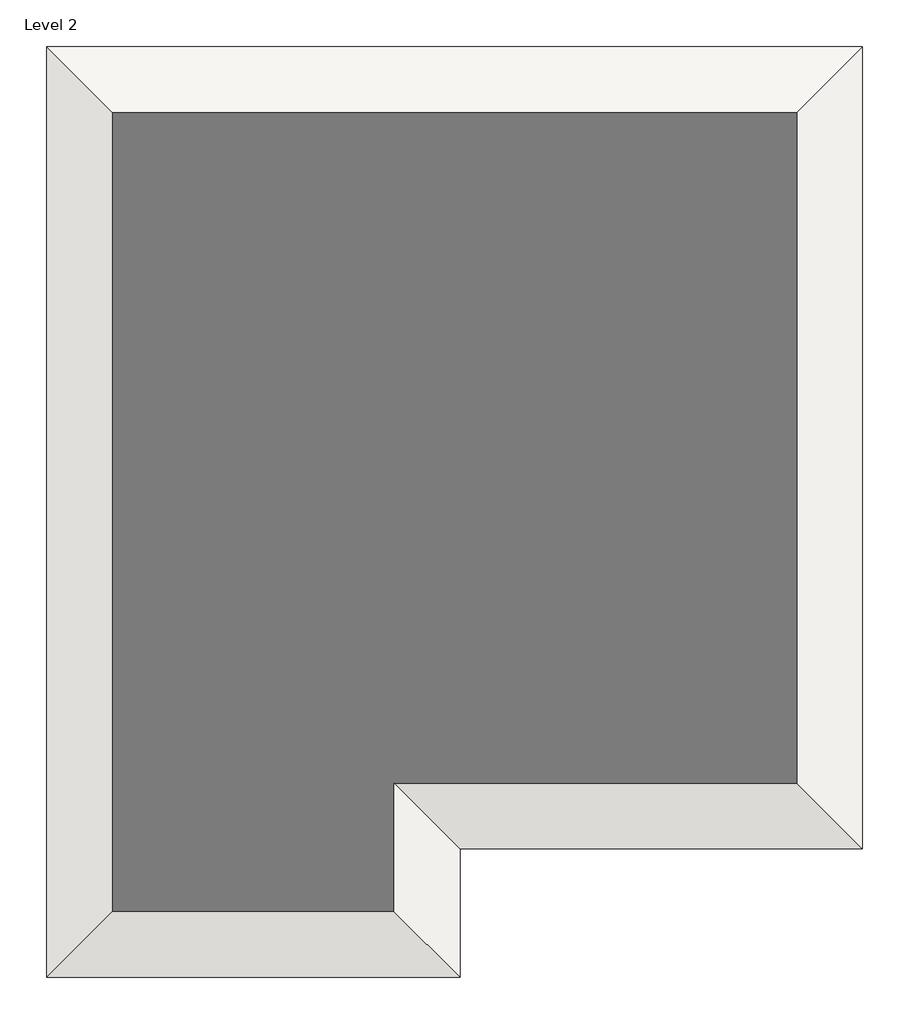
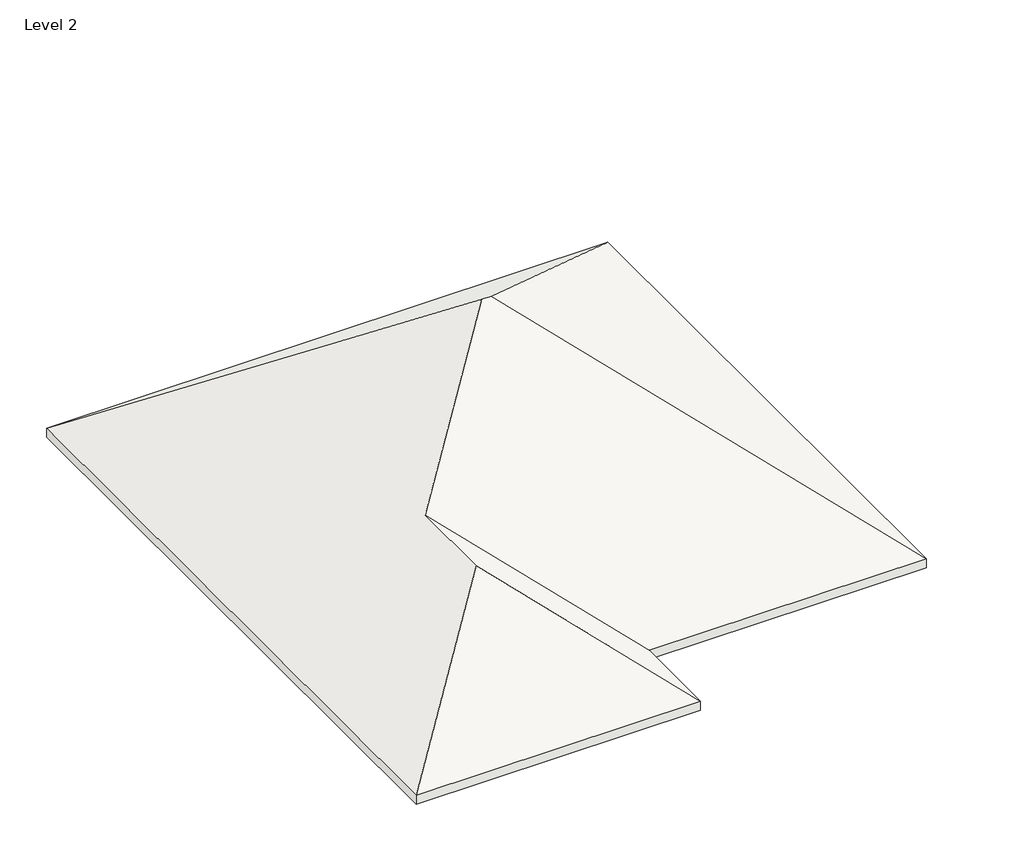
# One storey: 1 roof.
"""IFC4 building model written with IfcOpenShell, lengths in millimetres."""

from ifc_helpers import new_model, si_unit, origin, place, context, project, spatial, faceted_brep, element, save

model = new_model("IFC4")

# Units and contexts
model_context = context("Model", 3, world=origin())
ifc_project = project(units=[si_unit("LENGTHUNIT", "METRE", prefix="MILLI")], contexts=[model_context])

# Site, building, storey
site = spatial("IfcSite", under=ifc_project)
building = spatial("IfcBuilding", under=site)
storey = spatial("IfcBuildingStorey", under=building, Name="Level 2", Elevation=3048.0)

# Roof
placement = place(None, origin())
element("IfcRoof", 1, ObjectType="Wood Rafter 8\" - Asphalt Shingle - Insulated", at=placement, inside=storey, context=model_context, shape_type="Brep", body=[
    faceted_brep([(-9212.4392853, 5944.3049175, 8748.7125), (-1611.4892853, 13545.2549175, 3048.0), (-1611.4892853, -1656.6450825, 3048.0), (-17080.0892853, -4095.0450825, 3048.0), (-13162.1392853, -177.0950825, 5986.4625), (-9244.1892853, -4095.0450825, 3048.0), (-9479.1392853, 5944.3049175, 8748.7125), (-17080.0892853, 13545.2549175, 3048.0), (-9244.1892853, -1656.6450825, 3048.0), (-13162.1392853, 2261.3049175, 5986.4625), (-1611.4892853, 13545.2549175, 3313.90625), (-9212.4392853, 5944.3049175, 9014.61875), (-1611.4892853, -1656.6450825, 3313.90625), (-17080.0892853, -4095.0450825, 3313.90625), (-9244.1892853, -4095.0450825, 3313.90625), (-13162.1392853, -177.0950825, 6252.36875), (-17080.0892853, 13545.2549175, 3313.90625), (-9479.1392853, 5944.3049175, 9014.61875), (-9244.1892853, -1656.6450825, 3313.90625), (-13162.1392853, 2261.3049175, 6252.36875)], [[[0, 1, 2]], [[3, 4, 5]], [[1, 0, 6, 7]], [[8, 9, 6, 0, 2]], [[7, 6, 9, 4, 3]], [[8, 5, 4, 9]], [[10, 11, 12]], [[13, 14, 15]], [[10, 16, 17, 11]], [[18, 12, 11, 17, 19]], [[16, 13, 15, 19, 17]], [[14, 18, 19, 15]], [[7, 16, 10, 1]], [[3, 13, 16, 7]], [[5, 14, 13, 3]], [[8, 18, 14, 5]], [[2, 12, 18, 8]], [[1, 10, 12, 2]]]),
])

save(model, "model.ifc")

# Revit data of these elements
# Type "Wood Rafter 8\" - Asphalt Shingle - Insulated"
#   Assembly Code = "B1020"
#   Layers, outside or top first: 0' - 0 1/4" "Asphalt Shingle" (function 4); 0' - 0 5/8" "Plywood, Sheathing" (function 2); 0' - 7 1/2" "Structure, Wood Joist/Rafter Layer, Batt Insulation" (function 1)
# Element 1 (IfcRoof, "Wood Rafter 8\" - Asphalt Shingle - Insulated")
#   built-in parameter 1001705 = 29.5755 (stored number, unit not read)
#   built-in parameter 1001710 = 33615
#   Phase Created = New Construction
#   Materials on its faces: "Structure, Wood Joist/Rafter Layer, Batt Insulation", "Asphalt Shingle"
# Materials
#   "Asphalt Shingle": class "Generic", colour RGB 155 155 155, transparency 0, Description = "Asphalt roofing shingle", Cost = 0
#   "Plywood, Sheathing": class "Wood", colour RGB 212 179 113, transparency 0, Description = "Plywood, sheathing grade", Cost = 0
#   "Structure, Wood Joist/Rafter Layer, Batt Insulation": class "Wood", colour RGB 127 127 127, transparency 0, Description = "Wood framing, insulated", Cost = 0
